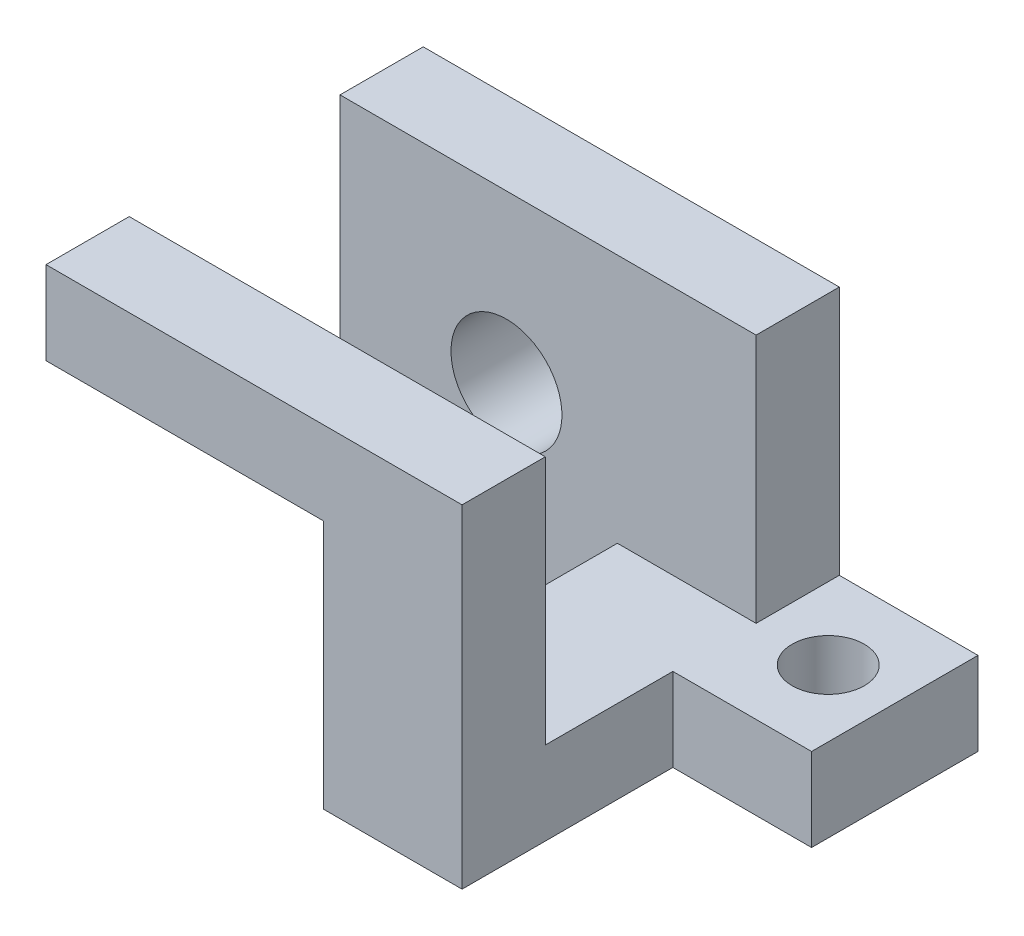
ISO-10303-21;
HEADER;
FILE_DESCRIPTION(('STEP AP214'),'2;1');
FILE_NAME('part.step','',(''),(''),'','','');
FILE_SCHEMA(('AUTOMOTIVE_DESIGN { 1 0 10303 214 1 1 1 1 }'));
ENDSEC;
DATA;
#1=APPLICATION_CONTEXT('core data for automotive mechanical design processes');
#2=APPLICATION_PROTOCOL_DEFINITION('international standard','automotive_design',2000,#1);
#3=PRODUCT_CONTEXT('',#1,'mechanical');
#4=PRODUCT('Part','Part','',(#3));
#5=PRODUCT_RELATED_PRODUCT_CATEGORY('part','',(#4));
#6=PRODUCT_DEFINITION_FORMATION('','',#4);
#7=PRODUCT_DEFINITION_CONTEXT('part definition',#1,'design');
#8=PRODUCT_DEFINITION('design','',#6,#7);
#9=PRODUCT_DEFINITION_SHAPE('','',#8);
#10=(LENGTH_UNIT() NAMED_UNIT(*) SI_UNIT(.MILLI.,.METRE.));
#11=(NAMED_UNIT(*) PLANE_ANGLE_UNIT() SI_UNIT($,.RADIAN.));
#12=(NAMED_UNIT(*) SI_UNIT($,.STERADIAN.) SOLID_ANGLE_UNIT());
#13=UNCERTAINTY_MEASURE_WITH_UNIT(LENGTH_MEASURE(1.E-05),#10,'distance_accuracy_value','');
#14=(GEOMETRIC_REPRESENTATION_CONTEXT(3) GLOBAL_UNCERTAINTY_ASSIGNED_CONTEXT((#13)) GLOBAL_UNIT_ASSIGNED_CONTEXT((#10,
#11,#12)) REPRESENTATION_CONTEXT('',''));
#15=CARTESIAN_POINT('',(0.,0.,0.));
#16=DIRECTION('',(0.,0.,1.));
#17=DIRECTION('',(1.,0.,0.));
#18=AXIS2_PLACEMENT_3D('',#15,#16,#17);
#19=CARTESIAN_POINT('',(-25.,0.,-15.));
#20=DIRECTION('',(0.,-1.,0.));
#21=DIRECTION('',(0.,0.,-1.));
#22=AXIS2_PLACEMENT_3D('',#19,#20,#21);
#23=PLANE('',#22);
#24=CARTESIAN_POINT('',(13.,0.,-53.));
#25=DIRECTION('',(0.,1.,0.));
#26=DIRECTION('',(0.,0.,1.));
#27=AXIS2_PLACEMENT_3D('',#24,#25,#26);
#28=CIRCLE('',#27,6.5);
#29=CARTESIAN_POINT('',(13.,0.,-46.5));
#30=VERTEX_POINT('',#29);
#31=EDGE_CURVE('E265',#30,#30,#28,.T.);
#32=ORIENTED_EDGE('',*,*,#31,.T.);
#33=EDGE_LOOP('',(#32));
#34=FACE_BOUND('',#33,.T.);
#35=DIRECTION('',(1.,0.,0.));
#36=VECTOR('',#35,1.);
#37=CARTESIAN_POINT('',(-25.,0.,0.));
#38=LINE('',#37,#36);
#39=CARTESIAN_POINT('',(-25.,0.,0.));
#40=VERTEX_POINT('',#39);
#41=CARTESIAN_POINT('',(0.,0.,0.));
#42=VERTEX_POINT('',#41);
#43=EDGE_CURVE('E220',#40,#42,#38,.T.);
#44=ORIENTED_EDGE('',*,*,#43,.F.);
#45=DIRECTION('',(0.,0.,1.));
#46=VECTOR('',#45,1.);
#47=CARTESIAN_POINT('',(-25.,0.,-15.));
#48=LINE('',#47,#46);
#49=CARTESIAN_POINT('',(-25.,0.,-53.));
#50=VERTEX_POINT('',#49);
#51=EDGE_CURVE('E47',#50,#40,#48,.T.);
#52=ORIENTED_EDGE('',*,*,#51,.F.);
#53=DIRECTION('',(1.,0.,0.));
#54=VECTOR('',#53,1.);
#55=CARTESIAN_POINT('',(0.,0.,-53.));
#56=LINE('',#55,#54);
#57=CARTESIAN_POINT('',(-75.,0.,-53.));
#58=VERTEX_POINT('',#57);
#59=EDGE_CURVE('E171',#58,#50,#56,.T.);
#60=ORIENTED_EDGE('',*,*,#59,.F.);
#61=DIRECTION('',(0.,0.,1.));
#62=VECTOR('',#61,1.);
#63=CARTESIAN_POINT('',(-75.,0.,-68.));
#64=LINE('',#63,#62);
#65=CARTESIAN_POINT('',(-75.,0.,-68.));
#66=VERTEX_POINT('',#65);
#67=EDGE_CURVE('E252',#66,#58,#64,.T.);
#68=ORIENTED_EDGE('',*,*,#67,.F.);
#69=DIRECTION('',(1.,0.,0.));
#70=VECTOR('',#69,1.);
#71=CARTESIAN_POINT('',(0.,0.,-68.));
#72=LINE('',#71,#70);
#73=CARTESIAN_POINT('',(25.,0.,-68.));
#74=VERTEX_POINT('',#73);
#75=EDGE_CURVE('E185',#66,#74,#72,.T.);
#76=ORIENTED_EDGE('',*,*,#75,.T.);
#77=DIRECTION('',(0.,0.,1.));
#78=VECTOR('',#77,1.);
#79=CARTESIAN_POINT('',(25.,0.,0.));
#80=LINE('',#79,#78);
#81=CARTESIAN_POINT('',(25.,0.,-38.));
#82=VERTEX_POINT('',#81);
#83=EDGE_CURVE('E177',#74,#82,#80,.T.);
#84=ORIENTED_EDGE('',*,*,#83,.T.);
#85=DIRECTION('',(1.,0.,0.));
#86=VECTOR('',#85,1.);
#87=CARTESIAN_POINT('',(0.,0.,-38.));
#88=LINE('',#87,#86);
#89=CARTESIAN_POINT('',(0.,0.,-38.));
#90=VERTEX_POINT('',#89);
#91=EDGE_CURVE('E195',#90,#82,#88,.T.);
#92=ORIENTED_EDGE('',*,*,#91,.F.);
#93=DIRECTION('',(0.,0.,1.));
#94=VECTOR('',#93,1.);
#95=CARTESIAN_POINT('',(0.,0.,-15.));
#96=LINE('',#95,#94);
#97=EDGE_CURVE('E226',#90,#42,#96,.T.);
#98=ORIENTED_EDGE('',*,*,#97,.T.);
#99=EDGE_LOOP('',(#44,#52,#60,#68,#76,#84,#92,#98));
#100=FACE_BOUND('',#99,.T.);
#101=ADVANCED_FACE('F41',(#34,#100),#23,.T.);
#102=CARTESIAN_POINT('',(-25.,45.,-15.));
#103=DIRECTION('',(-1.,0.,0.));
#104=DIRECTION('',(0.,-1.,0.));
#105=AXIS2_PLACEMENT_3D('',#102,#103,#104);
#106=PLANE('',#105);
#107=DIRECTION('',(0.,-1.,0.));
#108=VECTOR('',#107,1.);
#109=CARTESIAN_POINT('',(-25.,45.,-15.));
#110=LINE('',#109,#108);
#111=CARTESIAN_POINT('',(-25.,45.,-15.));
#112=VERTEX_POINT('',#111);
#113=CARTESIAN_POINT('',(-25.,15.,-15.));
#114=VERTEX_POINT('',#113);
#115=EDGE_CURVE('E229',#112,#114,#110,.T.);
#116=ORIENTED_EDGE('',*,*,#115,.T.);
#117=DIRECTION('',(0.,0.,-1.));
#118=VECTOR('',#117,1.);
#119=CARTESIAN_POINT('',(-25.,15.,0.));
#120=LINE('',#119,#118);
#121=CARTESIAN_POINT('',(-25.,15.,-53.));
#122=VERTEX_POINT('',#121);
#123=EDGE_CURVE('E60',#114,#122,#120,.T.);
#124=ORIENTED_EDGE('',*,*,#123,.T.);
#125=DIRECTION('',(0.,-1.,0.));
#126=VECTOR('',#125,1.);
#127=CARTESIAN_POINT('',(-25.,15.,-53.));
#128=LINE('',#127,#126);
#129=EDGE_CURVE('E215',#122,#50,#128,.T.);
#130=ORIENTED_EDGE('',*,*,#129,.T.);
#131=ORIENTED_EDGE('',*,*,#51,.T.);
#132=DIRECTION('',(0.,-1.,0.));
#133=VECTOR('',#132,1.);
#134=CARTESIAN_POINT('',(-25.,45.,0.));
#135=LINE('',#134,#133);
#136=CARTESIAN_POINT('',(-25.,45.,0.));
#137=VERTEX_POINT('',#136);
#138=EDGE_CURVE('E95',#137,#40,#135,.T.);
#139=ORIENTED_EDGE('',*,*,#138,.F.);
#140=DIRECTION('',(0.,0.,1.));
#141=VECTOR('',#140,1.);
#142=CARTESIAN_POINT('',(-25.,45.,-15.));
#143=LINE('',#142,#141);
#144=EDGE_CURVE('E63',#112,#137,#143,.T.);
#145=ORIENTED_EDGE('',*,*,#144,.F.);
#146=EDGE_LOOP('',(#116,#124,#130,#131,#139,#145));
#147=FACE_BOUND('',#146,.T.);
#148=ADVANCED_FACE('F278',(#147),#106,.T.);
#149=CARTESIAN_POINT('',(-75.,45.,-15.));
#150=DIRECTION('',(0.,-1.,0.));
#151=DIRECTION('',(1.,0.,0.));
#152=AXIS2_PLACEMENT_3D('',#149,#150,#151);
#153=PLANE('',#152);
#154=DIRECTION('',(1.,0.,0.));
#155=VECTOR('',#154,1.);
#156=CARTESIAN_POINT('',(-75.,45.,0.));
#157=LINE('',#156,#155);
#158=CARTESIAN_POINT('',(-75.,45.,0.));
#159=VERTEX_POINT('',#158);
#160=EDGE_CURVE('E239',#159,#137,#157,.T.);
#161=ORIENTED_EDGE('',*,*,#160,.F.);
#162=DIRECTION('',(0.,0.,1.));
#163=VECTOR('',#162,1.);
#164=CARTESIAN_POINT('',(-75.,45.,-15.));
#165=LINE('',#164,#163);
#166=CARTESIAN_POINT('',(-75.,45.,-15.));
#167=VERTEX_POINT('',#166);
#168=EDGE_CURVE('E241',#167,#159,#165,.T.);
#169=ORIENTED_EDGE('',*,*,#168,.F.);
#170=DIRECTION('',(1.,0.,0.));
#171=VECTOR('',#170,1.);
#172=CARTESIAN_POINT('',(-75.,45.,-15.));
#173=LINE('',#172,#171);
#174=EDGE_CURVE('E223',#167,#112,#173,.T.);
#175=ORIENTED_EDGE('',*,*,#174,.T.);
#176=ORIENTED_EDGE('',*,*,#144,.T.);
#177=EDGE_LOOP('',(#161,#169,#175,#176));
#178=FACE_BOUND('',#177,.T.);
#179=ADVANCED_FACE('F312',(#178),#153,.T.);
#180=CARTESIAN_POINT('',(-75.,60.,-15.));
#181=DIRECTION('',(-1.,0.,0.));
#182=DIRECTION('',(0.,0.,1.));
#183=AXIS2_PLACEMENT_3D('',#180,#181,#182);
#184=PLANE('',#183);
#185=DIRECTION('',(0.,-1.,0.));
#186=VECTOR('',#185,1.);
#187=CARTESIAN_POINT('',(-75.,60.,0.));
#188=LINE('',#187,#186);
#189=CARTESIAN_POINT('',(-75.,60.,0.));
#190=VERTEX_POINT('',#189);
#191=EDGE_CURVE('E237',#190,#159,#188,.T.);
#192=ORIENTED_EDGE('',*,*,#191,.F.);
#193=DIRECTION('',(0.,0.,1.));
#194=VECTOR('',#193,1.);
#195=CARTESIAN_POINT('',(-75.,60.,-15.));
#196=LINE('',#195,#194);
#197=CARTESIAN_POINT('',(-75.,60.,-15.));
#198=VERTEX_POINT('',#197);
#199=EDGE_CURVE('E248',#198,#190,#196,.T.);
#200=ORIENTED_EDGE('',*,*,#199,.F.);
#201=DIRECTION('',(0.,-1.,0.));
#202=VECTOR('',#201,1.);
#203=CARTESIAN_POINT('',(-75.,60.,-15.));
#204=LINE('',#203,#202);
#205=EDGE_CURVE('E225',#198,#167,#204,.T.);
#206=ORIENTED_EDGE('',*,*,#205,.T.);
#207=ORIENTED_EDGE('',*,*,#168,.T.);
#208=EDGE_LOOP('',(#192,#200,#206,#207));
#209=FACE_BOUND('',#208,.T.);
#210=ADVANCED_FACE('F429',(#209),#184,.T.);
#211=CARTESIAN_POINT('',(0.,60.,-15.));
#212=DIRECTION('',(0.,1.,0.));
#213=DIRECTION('',(-1.,0.,0.));
#214=AXIS2_PLACEMENT_3D('',#211,#212,#213);
#215=PLANE('',#214);
#216=DIRECTION('',(-1.,0.,0.));
#217=VECTOR('',#216,1.);
#218=CARTESIAN_POINT('',(0.,60.,0.));
#219=LINE('',#218,#217);
#220=CARTESIAN_POINT('',(0.,60.,0.));
#221=VERTEX_POINT('',#220);
#222=EDGE_CURVE('E231',#221,#190,#219,.T.);
#223=ORIENTED_EDGE('',*,*,#222,.F.);
#224=DIRECTION('',(0.,0.,1.));
#225=VECTOR('',#224,1.);
#226=CARTESIAN_POINT('',(0.,60.,-15.));
#227=LINE('',#226,#225);
#228=CARTESIAN_POINT('',(0.,60.,-15.));
#229=VERTEX_POINT('',#228);
#230=EDGE_CURVE('E246',#229,#221,#227,.T.);
#231=ORIENTED_EDGE('',*,*,#230,.F.);
#232=DIRECTION('',(-1.,0.,0.));
#233=VECTOR('',#232,1.);
#234=CARTESIAN_POINT('',(0.,60.,-15.));
#235=LINE('',#234,#233);
#236=EDGE_CURVE('E218',#229,#198,#235,.T.);
#237=ORIENTED_EDGE('',*,*,#236,.T.);
#238=ORIENTED_EDGE('',*,*,#199,.T.);
#239=EDGE_LOOP('',(#223,#231,#237,#238));
#240=FACE_BOUND('',#239,.T.);
#241=ADVANCED_FACE('F421',(#240),#215,.T.);
#242=CARTESIAN_POINT('',(0.,0.,-15.));
#243=DIRECTION('',(1.,0.,0.));
#244=DIRECTION('',(0.,0.,-1.));
#245=AXIS2_PLACEMENT_3D('',#242,#243,#244);
#246=PLANE('',#245);
#247=ORIENTED_EDGE('',*,*,#230,.T.);
#248=DIRECTION('',(0.,1.,0.));
#249=VECTOR('',#248,1.);
#250=CARTESIAN_POINT('',(0.,0.,0.));
#251=LINE('',#250,#249);
#252=EDGE_CURVE('E233',#42,#221,#251,.T.);
#253=ORIENTED_EDGE('',*,*,#252,.F.);
#254=ORIENTED_EDGE('',*,*,#97,.F.);
#255=DIRECTION('',(0.,-1.,0.));
#256=VECTOR('',#255,1.);
#257=CARTESIAN_POINT('',(0.,15.,-38.));
#258=LINE('',#257,#256);
#259=CARTESIAN_POINT('',(0.,15.,-38.));
#260=VERTEX_POINT('',#259);
#261=EDGE_CURVE('E207',#260,#90,#258,.T.);
#262=ORIENTED_EDGE('',*,*,#261,.F.);
#263=DIRECTION('',(0.,0.,-1.));
#264=VECTOR('',#263,1.);
#265=CARTESIAN_POINT('',(0.,15.,0.));
#266=LINE('',#265,#264);
#267=CARTESIAN_POINT('',(0.,15.,-15.));
#268=VERTEX_POINT('',#267);
#269=EDGE_CURVE('E200',#268,#260,#266,.T.);
#270=ORIENTED_EDGE('',*,*,#269,.F.);
#271=DIRECTION('',(0.,1.,0.));
#272=VECTOR('',#271,1.);
#273=CARTESIAN_POINT('',(0.,0.,-15.));
#274=LINE('',#273,#272);
#275=EDGE_CURVE('E99',#268,#229,#274,.T.);
#276=ORIENTED_EDGE('',*,*,#275,.T.);
#277=EDGE_LOOP('',(#247,#253,#254,#262,#270,#276));
#278=FACE_BOUND('',#277,.T.);
#279=ADVANCED_FACE('F291',(#278),#246,.T.);
#280=CARTESIAN_POINT('',(0.,0.,-15.));
#281=DIRECTION('',(0.,0.,1.));
#282=DIRECTION('',(1.,0.,0.));
#283=AXIS2_PLACEMENT_3D('',#280,#281,#282);
#284=PLANE('',#283);
#285=ORIENTED_EDGE('',*,*,#275,.F.);
#286=DIRECTION('',(-1.,0.,0.));
#287=VECTOR('',#286,1.);
#288=CARTESIAN_POINT('',(0.,15.,-15.));
#289=LINE('',#288,#287);
#290=EDGE_CURVE('E11',#268,#114,#289,.T.);
#291=ORIENTED_EDGE('',*,*,#290,.T.);
#292=ORIENTED_EDGE('',*,*,#115,.F.);
#293=ORIENTED_EDGE('',*,*,#174,.F.);
#294=ORIENTED_EDGE('',*,*,#205,.F.);
#295=ORIENTED_EDGE('',*,*,#236,.F.);
#296=EDGE_LOOP('',(#285,#291,#292,#293,#294,#295));
#297=FACE_BOUND('',#296,.T.);
#298=ADVANCED_FACE('F299',(#297),#284,.F.);
#299=CARTESIAN_POINT('',(0.,0.,0.));
#300=DIRECTION('',(0.,0.,1.));
#301=DIRECTION('',(1.,0.,0.));
#302=AXIS2_PLACEMENT_3D('',#299,#300,#301);
#303=PLANE('',#302);
#304=ORIENTED_EDGE('',*,*,#138,.T.);
#305=ORIENTED_EDGE('',*,*,#43,.T.);
#306=ORIENTED_EDGE('',*,*,#252,.T.);
#307=ORIENTED_EDGE('',*,*,#222,.T.);
#308=ORIENTED_EDGE('',*,*,#191,.T.);
#309=ORIENTED_EDGE('',*,*,#160,.T.);
#310=EDGE_LOOP('',(#304,#305,#306,#307,#308,#309));
#311=FACE_BOUND('',#310,.T.);
#312=ADVANCED_FACE('F293',(#311),#303,.T.);
#313=CARTESIAN_POINT('',(0.,15.,0.));
#314=DIRECTION('',(0.,1.,0.));
#315=DIRECTION('',(0.,0.,1.));
#316=AXIS2_PLACEMENT_3D('',#313,#314,#315);
#317=PLANE('',#316);
#318=CARTESIAN_POINT('',(13.,15.,-53.));
#319=DIRECTION('',(0.,1.,0.));
#320=DIRECTION('',(0.,0.,1.));
#321=AXIS2_PLACEMENT_3D('',#318,#319,#320);
#322=CIRCLE('',#321,6.5);
#323=CARTESIAN_POINT('',(13.,15.,-46.5));
#324=VERTEX_POINT('',#323);
#325=EDGE_CURVE('E42',#324,#324,#322,.T.);
#326=ORIENTED_EDGE('',*,*,#325,.F.);
#327=EDGE_LOOP('',(#326));
#328=FACE_BOUND('',#327,.T.);
#329=ORIENTED_EDGE('',*,*,#290,.F.);
#330=ORIENTED_EDGE('',*,*,#269,.T.);
#331=DIRECTION('',(1.,0.,0.));
#332=VECTOR('',#331,1.);
#333=CARTESIAN_POINT('',(0.,15.,-38.));
#334=LINE('',#333,#332);
#335=CARTESIAN_POINT('',(25.,15.,-38.));
#336=VERTEX_POINT('',#335);
#337=EDGE_CURVE('E203',#260,#336,#334,.T.);
#338=ORIENTED_EDGE('',*,*,#337,.T.);
#339=DIRECTION('',(0.,0.,1.));
#340=VECTOR('',#339,1.);
#341=CARTESIAN_POINT('',(25.,15.,0.));
#342=LINE('',#341,#340);
#343=CARTESIAN_POINT('',(25.,15.,-68.));
#344=VERTEX_POINT('',#343);
#345=EDGE_CURVE('E190',#344,#336,#342,.T.);
#346=ORIENTED_EDGE('',*,*,#345,.F.);
#347=DIRECTION('',(1.,0.,0.));
#348=VECTOR('',#347,1.);
#349=CARTESIAN_POINT('',(0.,15.,-68.));
#350=LINE('',#349,#348);
#351=CARTESIAN_POINT('',(0.,15.,-68.));
#352=VERTEX_POINT('',#351);
#353=EDGE_CURVE('E193',#352,#344,#350,.T.);
#354=ORIENTED_EDGE('',*,*,#353,.F.);
#355=DIRECTION('',(0.,0.,1.));
#356=VECTOR('',#355,1.);
#357=CARTESIAN_POINT('',(0.,15.,0.));
#358=LINE('',#357,#356);
#359=CARTESIAN_POINT('',(0.,15.,-53.));
#360=VERTEX_POINT('',#359);
#361=EDGE_CURVE('E176',#352,#360,#358,.T.);
#362=ORIENTED_EDGE('',*,*,#361,.T.);
#363=DIRECTION('',(1.,0.,0.));
#364=VECTOR('',#363,1.);
#365=CARTESIAN_POINT('',(0.,15.,-53.));
#366=LINE('',#365,#364);
#367=EDGE_CURVE('E194',#122,#360,#366,.T.);
#368=ORIENTED_EDGE('',*,*,#367,.F.);
#369=ORIENTED_EDGE('',*,*,#123,.F.);
#370=EDGE_LOOP('',(#329,#330,#338,#346,#354,#362,#368,#369));
#371=FACE_BOUND('',#370,.T.);
#372=ADVANCED_FACE('F282',(#328,#371),#317,.T.);
#373=CARTESIAN_POINT('',(25.,15.,0.));
#374=DIRECTION('',(1.,0.,0.));
#375=DIRECTION('',(0.,0.,-1.));
#376=AXIS2_PLACEMENT_3D('',#373,#374,#375);
#377=PLANE('',#376);
#378=ORIENTED_EDGE('',*,*,#83,.F.);
#379=DIRECTION('',(0.,-1.,0.));
#380=VECTOR('',#379,1.);
#381=CARTESIAN_POINT('',(25.,15.,-68.));
#382=LINE('',#381,#380);
#383=EDGE_CURVE('E214',#344,#74,#382,.T.);
#384=ORIENTED_EDGE('',*,*,#383,.F.);
#385=ORIENTED_EDGE('',*,*,#345,.T.);
#386=DIRECTION('',(0.,-1.,0.));
#387=VECTOR('',#386,1.);
#388=CARTESIAN_POINT('',(25.,15.,-38.));
#389=LINE('',#388,#387);
#390=EDGE_CURVE('E205',#336,#82,#389,.T.);
#391=ORIENTED_EDGE('',*,*,#390,.T.);
#392=EDGE_LOOP('',(#378,#384,#385,#391));
#393=FACE_BOUND('',#392,.T.);
#394=ADVANCED_FACE('F283',(#393),#377,.T.);
#395=CARTESIAN_POINT('',(0.,15.,-68.));
#396=DIRECTION('',(0.,0.,-1.));
#397=DIRECTION('',(-1.,0.,0.));
#398=AXIS2_PLACEMENT_3D('',#395,#396,#397);
#399=PLANE('',#398);
#400=CARTESIAN_POINT('',(-45.,30.,-68.));
#401=DIRECTION('',(0.,0.,-1.));
#402=DIRECTION('',(-1.,0.,0.));
#403=AXIS2_PLACEMENT_3D('',#400,#401,#402);
#404=CIRCLE('',#403,10.);
#405=CARTESIAN_POINT('',(-55.,30.,-68.));
#406=VERTEX_POINT('',#405);
#407=EDGE_CURVE('E251',#406,#406,#404,.T.);
#408=ORIENTED_EDGE('',*,*,#407,.F.);
#409=EDGE_LOOP('',(#408));
#410=FACE_BOUND('',#409,.T.);
#411=ORIENTED_EDGE('',*,*,#75,.F.);
#412=DIRECTION('',(0.,-1.,0.));
#413=VECTOR('',#412,1.);
#414=CARTESIAN_POINT('',(-75.,60.,-68.));
#415=LINE('',#414,#413);
#416=CARTESIAN_POINT('',(-75.,60.,-68.));
#417=VERTEX_POINT('',#416);
#418=EDGE_CURVE('E161',#417,#66,#415,.T.);
#419=ORIENTED_EDGE('',*,*,#418,.F.);
#420=DIRECTION('',(-1.,0.,0.));
#421=VECTOR('',#420,1.);
#422=CARTESIAN_POINT('',(0.,60.,-68.));
#423=LINE('',#422,#421);
#424=CARTESIAN_POINT('',(0.,60.,-68.));
#425=VERTEX_POINT('',#424);
#426=EDGE_CURVE('E152',#425,#417,#423,.T.);
#427=ORIENTED_EDGE('',*,*,#426,.F.);
#428=DIRECTION('',(0.,-1.,0.));
#429=VECTOR('',#428,1.);
#430=CARTESIAN_POINT('',(0.,60.,-68.));
#431=LINE('',#430,#429);
#432=EDGE_CURVE('E157',#425,#352,#431,.T.);
#433=ORIENTED_EDGE('',*,*,#432,.T.);
#434=ORIENTED_EDGE('',*,*,#353,.T.);
#435=ORIENTED_EDGE('',*,*,#383,.T.);
#436=EDGE_LOOP('',(#411,#419,#427,#433,#434,#435));
#437=FACE_BOUND('',#436,.T.);
#438=ADVANCED_FACE('F156',(#410,#437),#399,.T.);
#439=CARTESIAN_POINT('',(0.,15.,-38.));
#440=DIRECTION('',(0.,0.,-1.));
#441=DIRECTION('',(-1.,0.,0.));
#442=AXIS2_PLACEMENT_3D('',#439,#440,#441);
#443=PLANE('',#442);
#444=ORIENTED_EDGE('',*,*,#91,.T.);
#445=ORIENTED_EDGE('',*,*,#390,.F.);
#446=ORIENTED_EDGE('',*,*,#337,.F.);
#447=ORIENTED_EDGE('',*,*,#261,.T.);
#448=EDGE_LOOP('',(#444,#445,#446,#447));
#449=FACE_BOUND('',#448,.T.);
#450=ADVANCED_FACE('F289',(#449),#443,.F.);
#451=CARTESIAN_POINT('',(0.,60.,-68.));
#452=DIRECTION('',(-1.,0.,0.));
#453=DIRECTION('',(0.,0.,1.));
#454=AXIS2_PLACEMENT_3D('',#451,#452,#453);
#455=PLANE('',#454);
#456=ORIENTED_EDGE('',*,*,#361,.F.);
#457=ORIENTED_EDGE('',*,*,#432,.F.);
#458=DIRECTION('',(0.,0.,-1.));
#459=VECTOR('',#458,1.);
#460=CARTESIAN_POINT('',(0.,60.,-68.));
#461=LINE('',#460,#459);
#462=CARTESIAN_POINT('',(0.,60.,-53.));
#463=VERTEX_POINT('',#462);
#464=EDGE_CURVE('E164',#463,#425,#461,.T.);
#465=ORIENTED_EDGE('',*,*,#464,.F.);
#466=DIRECTION('',(0.,-1.,0.));
#467=VECTOR('',#466,1.);
#468=CARTESIAN_POINT('',(0.,60.,-53.));
#469=LINE('',#468,#467);
#470=EDGE_CURVE('E266',#463,#360,#469,.T.);
#471=ORIENTED_EDGE('',*,*,#470,.T.);
#472=EDGE_LOOP('',(#456,#457,#465,#471));
#473=FACE_BOUND('',#472,.T.);
#474=ADVANCED_FACE('F180',(#473),#455,.F.);
#475=CARTESIAN_POINT('',(-75.,60.,-68.));
#476=DIRECTION('',(1.,0.,0.));
#477=DIRECTION('',(0.,0.,-1.));
#478=AXIS2_PLACEMENT_3D('',#475,#476,#477);
#479=PLANE('',#478);
#480=ORIENTED_EDGE('',*,*,#67,.T.);
#481=DIRECTION('',(0.,-1.,0.));
#482=VECTOR('',#481,1.);
#483=CARTESIAN_POINT('',(-75.,60.,-53.));
#484=LINE('',#483,#482);
#485=CARTESIAN_POINT('',(-75.,60.,-53.));
#486=VERTEX_POINT('',#485);
#487=EDGE_CURVE('E184',#486,#58,#484,.T.);
#488=ORIENTED_EDGE('',*,*,#487,.F.);
#489=DIRECTION('',(0.,0.,1.));
#490=VECTOR('',#489,1.);
#491=CARTESIAN_POINT('',(-75.,60.,-68.));
#492=LINE('',#491,#490);
#493=EDGE_CURVE('E163',#417,#486,#492,.T.);
#494=ORIENTED_EDGE('',*,*,#493,.F.);
#495=ORIENTED_EDGE('',*,*,#418,.T.);
#496=EDGE_LOOP('',(#480,#488,#494,#495));
#497=FACE_BOUND('',#496,.T.);
#498=ADVANCED_FACE('F335',(#497),#479,.F.);
#499=CARTESIAN_POINT('',(0.,60.,-53.));
#500=DIRECTION('',(0.,0.,-1.));
#501=DIRECTION('',(-1.,0.,0.));
#502=AXIS2_PLACEMENT_3D('',#499,#500,#501);
#503=PLANE('',#502);
#504=CARTESIAN_POINT('',(-45.,30.,-53.));
#505=DIRECTION('',(0.,0.,-1.));
#506=DIRECTION('',(-1.,0.,0.));
#507=AXIS2_PLACEMENT_3D('',#504,#505,#506);
#508=CIRCLE('',#507,10.);
#509=CARTESIAN_POINT('',(-55.,30.,-53.));
#510=VERTEX_POINT('',#509);
#511=EDGE_CURVE('E249',#510,#510,#508,.T.);
#512=ORIENTED_EDGE('',*,*,#511,.T.);
#513=EDGE_LOOP('',(#512));
#514=FACE_BOUND('',#513,.T.);
#515=ORIENTED_EDGE('',*,*,#129,.F.);
#516=ORIENTED_EDGE('',*,*,#367,.T.);
#517=ORIENTED_EDGE('',*,*,#470,.F.);
#518=DIRECTION('',(1.,0.,0.));
#519=VECTOR('',#518,1.);
#520=CARTESIAN_POINT('',(0.,60.,-53.));
#521=LINE('',#520,#519);
#522=EDGE_CURVE('E168',#486,#463,#521,.T.);
#523=ORIENTED_EDGE('',*,*,#522,.F.);
#524=ORIENTED_EDGE('',*,*,#487,.T.);
#525=ORIENTED_EDGE('',*,*,#59,.T.);
#526=EDGE_LOOP('',(#515,#516,#517,#523,#524,#525));
#527=FACE_BOUND('',#526,.T.);
#528=ADVANCED_FACE('F274',(#514,#527),#503,.F.);
#529=CARTESIAN_POINT('',(0.,60.,0.));
#530=DIRECTION('',(0.,-1.,0.));
#531=DIRECTION('',(0.,0.,-1.));
#532=AXIS2_PLACEMENT_3D('',#529,#530,#531);
#533=PLANE('',#532);
#534=ORIENTED_EDGE('',*,*,#464,.T.);
#535=ORIENTED_EDGE('',*,*,#426,.T.);
#536=ORIENTED_EDGE('',*,*,#493,.T.);
#537=ORIENTED_EDGE('',*,*,#522,.T.);
#538=EDGE_LOOP('',(#534,#535,#536,#537));
#539=FACE_BOUND('',#538,.T.);
#540=ADVANCED_FACE('F169',(#539),#533,.F.);
#541=CARTESIAN_POINT('',(-45.,30.,0.));
#542=DIRECTION('',(0.,0.,-1.));
#543=DIRECTION('',(-1.,0.,0.));
#544=AXIS2_PLACEMENT_3D('',#541,#542,#543);
#545=CYLINDRICAL_SURFACE('',#544,10.);
#546=ORIENTED_EDGE('',*,*,#407,.T.);
#547=EDGE_LOOP('',(#546));
#548=FACE_BOUND('',#547,.T.);
#549=ORIENTED_EDGE('',*,*,#511,.F.);
#550=EDGE_LOOP('',(#549));
#551=FACE_BOUND('',#550,.T.);
#552=ADVANCED_FACE('F321',(#548,#551),#545,.F.);
#553=CARTESIAN_POINT('',(13.,0.,-53.));
#554=DIRECTION('',(0.,1.,0.));
#555=DIRECTION('',(0.,0.,1.));
#556=AXIS2_PLACEMENT_3D('',#553,#554,#555);
#557=CYLINDRICAL_SURFACE('',#556,6.5);
#558=ORIENTED_EDGE('',*,*,#325,.T.);
#559=EDGE_LOOP('',(#558));
#560=FACE_BOUND('',#559,.T.);
#561=ORIENTED_EDGE('',*,*,#31,.F.);
#562=EDGE_LOOP('',(#561));
#563=FACE_BOUND('',#562,.T.);
#564=ADVANCED_FACE('F317',(#560,#563),#557,.F.);
#565=CLOSED_SHELL('',(#101,#148,#179,#210,#241,#279,#298,#312,#372,#394,#438,#450,#474,#498,
#528,#540,#552,#564));
#566=MANIFOLD_SOLID_BREP('B2',#565);
#567=ADVANCED_BREP_SHAPE_REPRESENTATION('',(#18,#566),#14);
#568=SHAPE_DEFINITION_REPRESENTATION(#9,#567);
ENDSEC;
END-ISO-10303-21;
